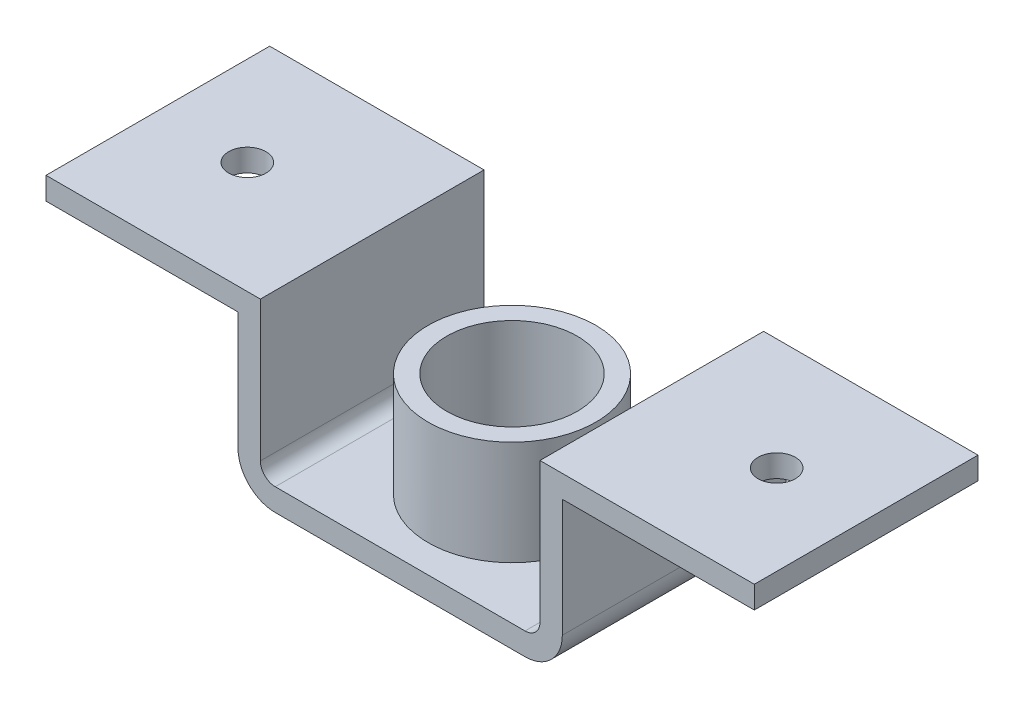
from build123d import *

# Parameters (mm, degrees)
Z_BRACKET_BODY_DEPTH        = 150
TUBE_BOSS_SKETCH_R          = 112.5
TUBE_BOSS_SKETCH_R_2        = 87.5
TUBE_BOSS_225X_175_DEPTH    = 140
CENTRE_HOLE_SKETCH_R        = 37.5
CENTRE_HOLE_75_DEPTH        = 140
FLANGE_HOLES_SKETCH_R       = 25
FLANGE_MOUNTING_HOLES_DEPTH = 140
BEND_FILLET_R20_R           = 20
BEND_FILLET_R50_R           = 50


with BuildPart() as part:
    # Bracket Profile Sketch → Z Bracket Body (new, symmetric)
    with BuildSketch(Plane.XY):
        Polygon((-475, 208), (-187.5, 208), (-187.5, 0), (187.5, 0), (187.5, 208), (475, 208), (475, 178), (217.5, 178), (217.5, -30), (-217.5, -30), (-217.5, 178), (-475, 178), align=None)
    extrude(amount=Z_BRACKET_BODY_DEPTH, both=True)

    # Tube Boss Sketch → Tube Boss Ø225xØ175 (add)
    with BuildSketch(Plane(origin=(0, 0, 0), x_dir=(1, 0, 0), z_dir=(0, 1, 0))):
        with Locations(Location((0, 0, 0), (0, 0, 90))):
            Circle(TUBE_BOSS_SKETCH_R)
        with Locations(Location((0, 0, 0), (0, 0, 270))):
            Circle(TUBE_BOSS_SKETCH_R_2, mode=Mode.SUBTRACT)
    extrude(amount=TUBE_BOSS_225X_175_DEPTH)

    # Centre Hole Sketch → Centre Hole Ø75 (cut)
    with BuildSketch(Plane(origin=(0, 0, 0), x_dir=(1, 0, 0), z_dir=(0, 1, 0))):
        with Locations(Location((0, 0, 0), (0, 0, 270))):
            Circle(CENTRE_HOLE_SKETCH_R)
    extrude(amount=-CENTRE_HOLE_75_DEPTH, mode=Mode.SUBTRACT)

    # Flange Holes Sketch → Flange Mounting Holes (cut)
    with BuildSketch(Plane(origin=(0, 208, 0), x_dir=(1, 0, 0), z_dir=(0, 1, 0))):
        with Locations(Location((-355, 0, 0), (0, 0, 270))):
            Circle(FLANGE_HOLES_SKETCH_R)
        with Locations(Location((355, 0, 0), (0, 0, 270))):
            Circle(FLANGE_HOLES_SKETCH_R)
    extrude(amount=-FLANGE_MOUNTING_HOLES_DEPTH, mode=Mode.SUBTRACT)

    # Bend Fillet R20
    bend_fillet_r20_edges = [part.edges().sort_by_distance(p)[0] for p in [
        (-187.5, 0, 0),
        (187.5, 0, 0),
    ]]
    fillet(bend_fillet_r20_edges, radius=BEND_FILLET_R20_R)

    # Bend Fillet R50
    bend_fillet_r50_edges = [part.edges().sort_by_distance(p)[0] for p in [
        (217.5, -30, 0),
        (-217.5, -30, 0),
    ]]
    fillet(bend_fillet_r50_edges, radius=BEND_FILLET_R50_R)


solid = part.part
